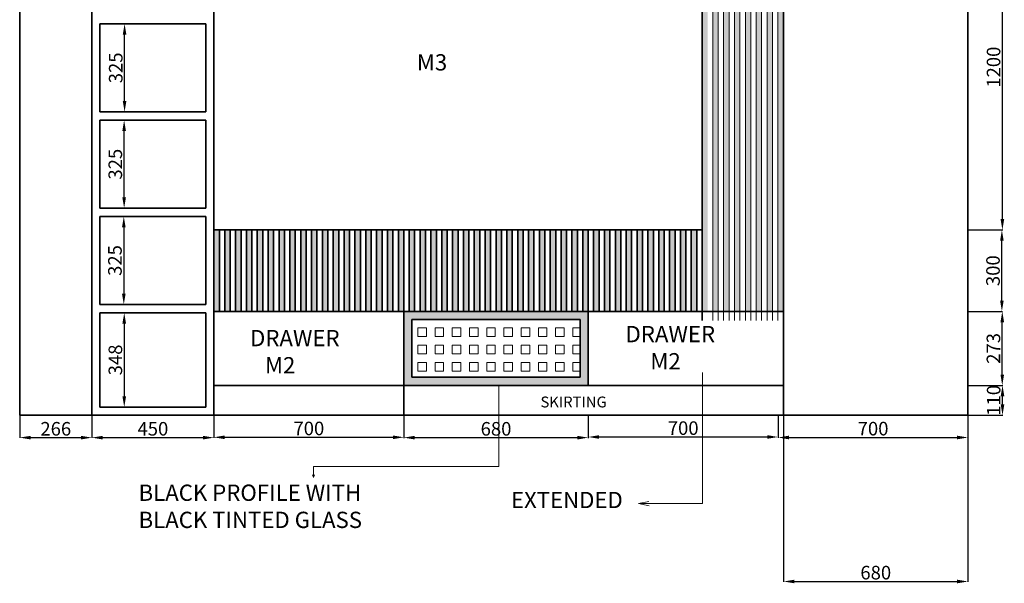
# Model space of a CAD drawing. Units: millimetres. Extents: x 11439 to 24661, y -4767 to -6.
# Tile 3 of 5: x 18965 to 22595, y -4767 to -2690. Entities that reach past the tile are written whole.
import ezdxf

# ---------------------------------------------------------------- set-up
doc = ezdxf.new("R2010")
doc.units = ezdxf.units.MM
for name, color, linetype, lineweight in [('A-ANNO-DIMS', 2, 'Continuous', 18), ('A-ANNO-TEXT', 3, 'Continuous', 18), ('A-FURN', 7, 'Continuous', 35), ('A-FURN-PATT', 8, 'Continuous', 13)]:
    doc.layers.add(name, color=color, linetype=linetype, lineweight=lineweight)
doc.styles.get("Standard").update_dxf_attribs({"font": 'arial.ttf'})
doc.dimstyles.new('ISO-25', dxfattribs={"dimtxt": 50, "dimasz": 40, "dimexe": 1.25, "dimexo": 0.625, "dimtad": 1, "dimtxsty": 'Standard', "dimcen": 2.5, "dimadec": 0, "dimazin": 0, "dimtfac": 1, "dimtmove": 0, "dimatfit": 3, "dimfxl": 1, "dimarcsym": 0})

# ---------------------------------------------------------------- blocks, each defined once
blk = doc.blocks.new('*D31')
at = {"layer": 'A-ANNO-DIMS', "color": 0, "lineweight": -2, "transparency": 16777216}
for p, q in [((18964.8, -4148.3), (18964.8, -4231.3)), ((19230.8, -4148.3), (19230.8, -4231.3)), ((19004.8, -4230), (19190.8, -4230))]:
    blk.add_line(p, q, dxfattribs=at)
at = {"layer": 'A-ANNO-DIMS', "color": 0, "transparency": 16777216}
for points in [[(19004.8, -4223.4), (19004.8, -4236.7), (18964.8, -4230)], [(19190.8, -4223.4), (19190.8, -4236.7), (19230.8, -4230)]]:
    blk.add_solid(points, dxfattribs=at)
at = {"layer": 'Defpoints', "color": 0, "transparency": 16777216}
for p in [(18964.8, -4147.7), (19230.8, -4147.7), (19230.8, -4230)]:
    blk.add_point(p, dxfattribs=at)
at = {"layer": 'A-ANNO-DIMS', "color": 0, "transparency": 16777216, "insert": (19097.8, -4203.9), "char_height": 50, "attachment_point": 5}
blk.add_mtext('266', dxfattribs=at)
blk = doc.blocks.new('*D32')
at = {"layer": 'A-ANNO-DIMS', "color": 0, "lineweight": -2, "transparency": 16777216}
for p, q in [((19230.8, -4148.3), (19230.8, -4231.3)), ((19680.8, -4148.3), (19680.8, -4231.3)), ((19270.8, -4230), (19640.8, -4230))]:
    blk.add_line(p, q, dxfattribs=at)
at = {"layer": 'A-ANNO-DIMS', "color": 0, "transparency": 16777216}
for points in [[(19270.8, -4223.4), (19270.8, -4236.7), (19230.8, -4230)], [(19640.8, -4223.4), (19640.8, -4236.7), (19680.8, -4230)]]:
    blk.add_solid(points, dxfattribs=at)
at = {"layer": 'Defpoints', "color": 0, "transparency": 16777216}
for p in [(19230.8, -4147.7), (19680.8, -4147.7), (19680.8, -4230)]:
    blk.add_point(p, dxfattribs=at)
at = {"layer": 'A-ANNO-DIMS', "color": 0, "transparency": 16777216, "insert": (19455.8, -4203.9), "char_height": 50, "attachment_point": 5}
blk.add_mtext('450', dxfattribs=at)
blk = doc.blocks.new('*D33')
at = {"layer": 'A-ANNO-DIMS', "color": 0, "lineweight": -2, "transparency": 16777216}
for p, q in [((19680.8, -4148.3), (19680.8, -4230.1)), ((20380.8, -4148.3), (20380.8, -4230.1)), ((19720.8, -4228.8), (20340.8, -4228.8))]:
    blk.add_line(p, q, dxfattribs=at)
at = {"layer": 'A-ANNO-DIMS', "color": 0, "transparency": 16777216}
for points in [[(19720.8, -4222.2), (19720.8, -4235.5), (19680.8, -4228.8)], [(20340.8, -4222.2), (20340.8, -4235.5), (20380.8, -4228.8)]]:
    blk.add_solid(points, dxfattribs=at)
at = {"layer": 'Defpoints', "color": 0, "transparency": 16777216}
for p in [(19680.8, -4147.7), (20380.8, -4147.7), (20380.8, -4228.8)]:
    blk.add_point(p, dxfattribs=at)
at = {"layer": 'A-ANNO-DIMS', "color": 0, "transparency": 16777216, "insert": (20030.8, -4202.7), "char_height": 50, "attachment_point": 5}
blk.add_mtext('700', dxfattribs=at)
blk = doc.blocks.new('*D34')
at = {"layer": 'A-ANNO-DIMS', "color": 0, "lineweight": -2, "transparency": 16777216}
for p, q in [((20380.8, -4148.3), (20380.8, -4231.4)), ((21060.8, -4148.3), (21060.8, -4231.4)), ((20420.8, -4230.1), (21020.8, -4230.1))]:
    blk.add_line(p, q, dxfattribs=at)
at = {"layer": 'A-ANNO-DIMS', "color": 0, "transparency": 16777216}
for points in [[(20420.8, -4223.5), (20420.8, -4236.8), (20380.8, -4230.1)], [(21020.8, -4223.5), (21020.8, -4236.8), (21060.8, -4230.1)]]:
    blk.add_solid(points, dxfattribs=at)
at = {"layer": 'Defpoints', "color": 0, "transparency": 16777216}
for p in [(20380.8, -4147.7), (21060.8, -4147.7), (21060.8, -4230.1)]:
    blk.add_point(p, dxfattribs=at)
at = {"layer": 'A-ANNO-DIMS', "color": 0, "transparency": 16777216, "insert": (20720.8, -4204), "char_height": 50, "attachment_point": 5}
blk.add_mtext('680', dxfattribs=at)
blk = doc.blocks.new('*D21')
at = {"layer": 'A-ANNO-DIMS', "color": 0, "lineweight": -2, "transparency": 16777216}
for p, q in [((21060.8, -4148.3), (21060.8, -4228.9)), ((21760.8, -4148.3), (21760.8, -4228.9)), ((21100.8, -4227.7), (21720.8, -4227.7))]:
    blk.add_line(p, q, dxfattribs=at)
at = {"layer": 'A-ANNO-DIMS', "color": 0, "transparency": 16777216}
for points in [[(21100.8, -4221), (21100.8, -4234.4), (21060.8, -4227.7)], [(21720.8, -4221), (21720.8, -4234.4), (21760.8, -4227.7)]]:
    blk.add_solid(points, dxfattribs=at)
at = {"layer": 'Defpoints', "color": 0, "transparency": 16777216}
for p in [(21060.8, -4147.7), (21760.8, -4147.7), (21760.8, -4227.7)]:
    blk.add_point(p, dxfattribs=at)
at = {"layer": 'A-ANNO-DIMS', "color": 0, "transparency": 16777216, "insert": (21410.8, -4201.5), "char_height": 50, "attachment_point": 5}
blk.add_mtext('700', dxfattribs=at)
blk = doc.blocks.new('*D35')
at = {"layer": 'A-ANNO-DIMS', "color": 0, "lineweight": -2, "transparency": 16777216}
for p, q in [((21760.8, -4148.3), (21760.8, -4230.8)), ((22460.8, -4148.3), (22460.8, -4230.8)), ((21800.8, -4229.6), (22420.8, -4229.6))]:
    blk.add_line(p, q, dxfattribs=at)
at = {"layer": 'A-ANNO-DIMS', "color": 0, "transparency": 16777216}
for points in [[(21800.8, -4222.9), (21800.8, -4236.3), (21760.8, -4229.6)], [(22420.8, -4222.9), (22420.8, -4236.3), (22460.8, -4229.6)]]:
    blk.add_solid(points, dxfattribs=at)
at = {"layer": 'Defpoints', "color": 0, "transparency": 16777216}
for p in [(21760.8, -4147.7), (22460.8, -4147.7), (22460.8, -4229.6)]:
    blk.add_point(p, dxfattribs=at)
at = {"layer": 'A-ANNO-DIMS', "color": 0, "transparency": 16777216, "insert": (22110.8, -4203.4), "char_height": 50, "attachment_point": 5}
blk.add_mtext('700', dxfattribs=at)
blk = doc.blocks.new('*D22')
at = {"layer": 'A-ANNO-DIMS', "color": 0, "lineweight": -2, "transparency": 16777216}
for p, q in [((22461.4, -4037.7), (22589.2, -4037.7)), ((22588, -4107.7), (22588, -4077.7)), ((22461.4, -4147.7), (22589.2, -4147.7))]:
    blk.add_line(p, q, dxfattribs=at)
at = {"layer": 'A-ANNO-DIMS', "color": 0, "transparency": 16777216}
for points in [[(22581.3, -4077.7), (22594.7, -4077.7), (22588, -4037.7)], [(22581.3, -4107.7), (22594.7, -4107.7), (22588, -4147.7)]]:
    blk.add_solid(points, dxfattribs=at)
at = {"layer": 'Defpoints', "color": 0, "transparency": 16777216}
for p in [(22460.8, -4037.7), (22588, -4037.7), (22460.8, -4147.7)]:
    blk.add_point(p, dxfattribs=at)
at = {"layer": 'A-ANNO-DIMS', "color": 0, "transparency": 16777216, "insert": (22561.8, -4092.7), "char_height": 50, "attachment_point": 5, "rotation": 90}
blk.add_mtext('110', dxfattribs=at)
blk = doc.blocks.new('*D26')
at = {"layer": 'A-ANNO-DIMS', "color": 0, "lineweight": -2, "transparency": 16777216}
for p, q in [((22461.4, -3764.7), (22588.4, -3764.7)), ((22587.1, -3997.7), (22587.1, -3804.7)), ((22461.4, -4037.7), (22588.4, -4037.7))]:
    blk.add_line(p, q, dxfattribs=at)
at = {"layer": 'A-ANNO-DIMS', "color": 0, "transparency": 16777216}
for points in [[(22580.5, -3804.7), (22593.8, -3804.7), (22587.1, -3764.7)], [(22580.5, -3997.7), (22593.8, -3997.7), (22587.1, -4037.7)]]:
    blk.add_solid(points, dxfattribs=at)
at = {"layer": 'Defpoints', "color": 0, "transparency": 16777216}
for p in [(22460.8, -3764.7), (22587.1, -3764.7), (22460.8, -4037.7)]:
    blk.add_point(p, dxfattribs=at)
at = {"layer": 'A-ANNO-DIMS', "color": 0, "transparency": 16777216, "insert": (22561, -3901.2), "char_height": 50, "attachment_point": 5, "rotation": 90}
blk.add_mtext('273', dxfattribs=at)
blk = doc.blocks.new('*D27')
at = {"layer": 'A-ANNO-DIMS', "color": 0, "lineweight": -2, "transparency": 16777216}
for p, q in [((22461.4, -3464.7), (22586.9, -3464.7)), ((22585.7, -3724.7), (22585.7, -3504.7)), ((22461.4, -3764.7), (22586.9, -3764.7))]:
    blk.add_line(p, q, dxfattribs=at)
at = {"layer": 'A-ANNO-DIMS', "color": 0, "transparency": 16777216}
for points in [[(22579, -3504.7), (22592.4, -3504.7), (22585.7, -3464.7)], [(22579, -3724.7), (22592.4, -3724.7), (22585.7, -3764.7)]]:
    blk.add_solid(points, dxfattribs=at)
at = {"layer": 'Defpoints', "color": 0, "transparency": 16777216}
for p in [(22460.8, -3464.7), (22585.7, -3464.7), (22460.8, -3764.7)]:
    blk.add_point(p, dxfattribs=at)
at = {"layer": 'A-ANNO-DIMS', "color": 0, "transparency": 16777216, "insert": (22559.5, -3614.7), "char_height": 50, "attachment_point": 5, "rotation": 90}
blk.add_mtext('300', dxfattribs=at)
blk = doc.blocks.new('*D28')
at = {"layer": 'A-ANNO-DIMS', "color": 0, "lineweight": -2, "transparency": 16777216}
for p, q in [((22461.4, -2264.7), (22588.9, -2264.7)), ((22587.6, -3424.7), (22587.6, -2304.7)), ((22461.4, -3464.7), (22588.9, -3464.7))]:
    blk.add_line(p, q, dxfattribs=at)
at = {"layer": 'A-ANNO-DIMS', "color": 0, "transparency": 16777216}
for points in [[(22581, -2304.7), (22594.3, -2304.7), (22587.6, -2264.7)], [(22581, -3424.7), (22594.3, -3424.7), (22587.6, -3464.7)]]:
    blk.add_solid(points, dxfattribs=at)
at = {"layer": 'Defpoints', "color": 0, "transparency": 16777216}
for p in [(22460.8, -2264.7), (22587.6, -2264.7), (22460.8, -3464.7)]:
    blk.add_point(p, dxfattribs=at)
at = {"layer": 'A-ANNO-DIMS', "color": 0, "transparency": 16777216, "insert": (22561.5, -2864.7), "char_height": 50, "attachment_point": 5, "rotation": 90}
blk.add_mtext('1200', dxfattribs=at)
blk = doc.blocks.new('*D37')
at = {"layer": 'A-ANNO-DIMS', "color": 0, "lineweight": -2, "transparency": 16777216}
for p, q in [((19455.1, -3769.7), (19348.9, -3769.7)), ((19350.2, -3809.7), (19350.2, -4077.7)), ((19455.1, -4117.7), (19348.9, -4117.7))]:
    blk.add_line(p, q, dxfattribs=at)
at = {"layer": 'A-ANNO-DIMS', "color": 0, "transparency": 16777216}
for points in [[(19343.5, -3809.7), (19356.8, -3809.7), (19350.2, -3769.7)], [(19343.5, -4077.7), (19356.8, -4077.7), (19350.2, -4117.7)]]:
    blk.add_solid(points, dxfattribs=at)
at = {"layer": 'Defpoints', "color": 0, "transparency": 16777216}
for p in [(19455.8, -3769.7), (19350.2, -4117.7), (19455.8, -4117.7)]:
    blk.add_point(p, dxfattribs=at)
at = {"layer": 'A-ANNO-DIMS', "color": 0, "transparency": 16777216, "insert": (19324, -3943.7), "char_height": 50, "attachment_point": 5, "rotation": 90}
blk.add_mtext('348', dxfattribs=at)
blk = doc.blocks.new('*D38')
at = {"layer": 'A-ANNO-DIMS', "color": 0, "lineweight": -2, "transparency": 16777216}
for p, q in [((19261.4, -3414.7), (19349.8, -3414.7)), ((19348.6, -3454.7), (19348.6, -3699.7)), ((19261.4, -3739.7), (19349.8, -3739.7))]:
    blk.add_line(p, q, dxfattribs=at)
at = {"layer": 'A-ANNO-DIMS', "color": 0, "transparency": 16777216}
for points in [[(19341.9, -3454.7), (19355.3, -3454.7), (19348.6, -3414.7)], [(19341.9, -3699.7), (19355.3, -3699.7), (19348.6, -3739.7)]]:
    blk.add_solid(points, dxfattribs=at)
at = {"layer": 'Defpoints', "color": 0, "transparency": 16777216}
for p in [(19260.8, -3414.7), (19260.8, -3739.7), (19348.6, -3739.7)]:
    blk.add_point(p, dxfattribs=at)
at = {"layer": 'A-ANNO-DIMS', "color": 0, "transparency": 16777216, "insert": (19322.4, -3577.2), "char_height": 50, "attachment_point": 5, "rotation": 90}
blk.add_mtext('325', dxfattribs=at)
blk = doc.blocks.new('*D39')
at = {"layer": 'A-ANNO-DIMS', "color": 0, "lineweight": -2, "transparency": 16777216}
for p, q in [((19261.4, -3059.7), (19351.1, -3059.7)), ((19349.8, -3344.7), (19349.8, -3099.7)), ((19261.4, -3384.7), (19351.1, -3384.7))]:
    blk.add_line(p, q, dxfattribs=at)
at = {"layer": 'A-ANNO-DIMS', "color": 0, "transparency": 16777216}
for points in [[(19343.2, -3099.7), (19356.5, -3099.7), (19349.8, -3059.7)], [(19343.2, -3344.7), (19356.5, -3344.7), (19349.8, -3384.7)]]:
    blk.add_solid(points, dxfattribs=at)
at = {"layer": 'Defpoints', "color": 0, "transparency": 16777216}
for p in [(19260.8, -3059.7), (19349.8, -3059.7), (19260.8, -3384.7)]:
    blk.add_point(p, dxfattribs=at)
at = {"layer": 'A-ANNO-DIMS', "color": 0, "transparency": 16777216, "insert": (19323.7, -3222.2), "char_height": 50, "attachment_point": 5, "rotation": 90}
blk.add_mtext('325', dxfattribs=at)
blk = doc.blocks.new('*D40')
at = {"layer": 'A-ANNO-DIMS', "color": 0, "lineweight": -2, "transparency": 16777216}
for p, q in [((19261.4, -2704.7), (19352.7, -2704.7)), ((19351.5, -2989.7), (19351.5, -2744.7)), ((19261.4, -3029.7), (19352.7, -3029.7))]:
    blk.add_line(p, q, dxfattribs=at)
at = {"layer": 'A-ANNO-DIMS', "color": 0, "transparency": 16777216}
for points in [[(19344.8, -2744.7), (19358.1, -2744.7), (19351.5, -2704.7)], [(19344.8, -2989.7), (19358.1, -2989.7), (19351.5, -3029.7)]]:
    blk.add_solid(points, dxfattribs=at)
at = {"layer": 'Defpoints', "color": 0, "transparency": 16777216}
for p in [(19260.8, -2704.7), (19351.5, -2704.7), (19260.8, -3029.7)]:
    blk.add_point(p, dxfattribs=at)
at = {"layer": 'A-ANNO-DIMS', "color": 0, "transparency": 16777216, "insert": (19325.3, -2867.2), "char_height": 50, "attachment_point": 5, "rotation": 90}
blk.add_mtext('325', dxfattribs=at)
blk = doc.blocks.new('SHELF-COMPARTMENT')
for p, q in [((0, 325), (390, 325)), ((0, 0), (0, 325)), ((390, 0), (390, 325)), ((0, 0), (390, 0))]:
    blk.add_line(p, q)
blk = doc.blocks.new('DRAWER-GLASS-FRONT')
for p, q in [((0, 213), (620, 213)), ((0, 0), (0, 213)), ((620, 0), (620, 213)), ((0, 0), (620, 0))]:
    blk.add_line(p, q)
blk = doc.blocks.new('*D59')
at = {"layer": 'A-ANNO-DIMS', "color": 0, "lineweight": -2, "transparency": 16777216}
for p, q in [((21780.8, -4148.3), (21780.8, -4761.5)), ((22460.8, -4148.3), (22460.8, -4761.5)), ((21820.8, -4760.3), (22420.8, -4760.3))]:
    blk.add_line(p, q, dxfattribs=at)
at = {"layer": 'A-ANNO-DIMS', "color": 0, "transparency": 16777216}
for points in [[(21820.8, -4753.6), (21820.8, -4766.9), (21780.8, -4760.3)], [(22420.8, -4753.6), (22420.8, -4766.9), (22460.8, -4760.3)]]:
    blk.add_solid(points, dxfattribs=at)
at = {"layer": 'Defpoints', "color": 0, "transparency": 16777216}
for p in [(21780.8, -4147.7), (22460.8, -4147.7), (22460.8, -4760.3)]:
    blk.add_point(p, dxfattribs=at)
at = {"layer": 'A-ANNO-DIMS', "color": 0, "transparency": 16777216, "insert": (22120.8, -4734.1), "char_height": 50, "attachment_point": 5}
blk.add_mtext('680', dxfattribs=at)

msp = doc.modelspace()

# ---------------------------------------------------------------- hatches: boundary and pattern name
at = {"layer": 'A-FURN-PATT'}
h = msp.add_hatch(color=256, dxfattribs=at)
h.dxf.hatch_style = 1
h.paths.add_polyline_path([(19700.761, -3464.684), (19680.761, -3464.684), (19680.761, -3764.684), (19700.761, -3764.684)])
h.paths.add_polyline_path([(19740.761, -3464.684), (19720.761, -3464.684), (19720.761, -3764.684), (19740.761, -3764.684)])
h.paths.add_polyline_path([(19780.761, -3464.684), (19760.761, -3464.684), (19760.761, -3764.684), (19780.761, -3764.684)])
h.paths.add_polyline_path([(19800.761, -3764.684), (19820.761, -3764.684), (19820.761, -3464.684), (19800.761, -3464.684)])
h.paths.add_polyline_path([(19860.761, -3464.684), (19840.761, -3464.684), (19840.761, -3764.684), (19860.761, -3764.684)])
h.paths.add_polyline_path([(19900.761, -3464.684), (19880.761, -3464.684), (19880.761, -3764.684), (19900.761, -3764.684)])
h.paths.add_polyline_path([(19940.761, -3464.684), (19920.761, -3464.684), (19920.761, -3764.684), (19940.761, -3764.684)])
h.paths.add_polyline_path([(19960.761, -3764.684), (19980.761, -3764.684), (19980.761, -3464.684), (19960.761, -3464.684)])
h.paths.add_polyline_path([(20020.761, -3464.684), (20000.761, -3464.684), (20000.761, -3764.684), (20020.761, -3764.684)])
h.paths.add_polyline_path([(20040.761, -3764.684), (20060.761, -3764.684), (20060.761, -3464.684), (20040.761, -3464.684)])
h.paths.add_polyline_path([(20080.761, -3764.684), (20100.761, -3764.684), (20100.761, -3464.684), (20080.761, -3464.684)])
h.paths.add_polyline_path([(20140.761, -3464.684), (20120.761, -3464.684), (20120.761, -3764.684), (20140.761, -3764.684)])
h.paths.add_polyline_path([(20160.761, -3764.684), (20180.761, -3764.684), (20180.761, -3464.684), (20160.761, -3464.684)])
h.paths.add_polyline_path([(20220.761, -3464.684), (20200.761, -3464.684), (20200.761, -3764.684), (20220.761, -3764.684)])
h.paths.add_polyline_path([(20240.761, -3764.684), (20260.761, -3764.684), (20260.761, -3464.684), (20240.761, -3464.684)])
h.paths.add_polyline_path([(20300.761, -3464.684), (20280.761, -3464.684), (20280.761, -3764.684), (20300.761, -3764.684)])
h.paths.add_polyline_path([(20340.761, -3464.684), (20320.761, -3464.684), (20320.761, -3764.684), (20340.761, -3764.684)])
h.paths.add_polyline_path([(20360.761, -3764.684), (20380.761, -3764.684), (20380.761, -3464.684), (20360.761, -3464.684)])
h.paths.add_polyline_path([(20400.761, -3764.684), (20420.761, -3764.684), (20420.761, -3464.684), (20400.761, -3464.684)])
h.paths.add_polyline_path([(20440.761, -3764.684), (20460.761, -3764.684), (20460.761, -3464.684), (20440.761, -3464.684)])
h.paths.add_polyline_path([(20480.761, -3764.684), (20500.761, -3764.684), (20500.761, -3464.684), (20480.761, -3464.684)])
h.paths.add_polyline_path([(20520.761, -3764.684), (20540.761, -3764.684), (20540.761, -3464.684), (20520.761, -3464.684)])
h.paths.add_polyline_path([(20560.761, -3764.684), (20580.761, -3764.684), (20580.761, -3464.684), (20560.761, -3464.684)])
h.paths.add_polyline_path([(20600.761, -3764.684), (20620.761, -3764.684), (20620.761, -3464.684), (20600.761, -3464.684)])
h.paths.add_polyline_path([(20660.761, -3464.684), (20640.761, -3464.684), (20640.761, -3764.684), (20660.761, -3764.684)])
h.paths.add_polyline_path([(20680.761, -3764.684), (20700.761, -3764.684), (20700.761, -3464.684), (20680.761, -3464.684)])
h.paths.add_polyline_path([(20740.761, -3464.684), (20720.761, -3464.684), (20720.761, -3764.684), (20740.761, -3764.684)])
h.paths.add_polyline_path([(20760.761, -3764.684), (20780.761, -3764.684), (20780.761, -3464.684), (20760.761, -3464.684)])
h.paths.add_polyline_path([(20800.761, -3764.684), (20820.761, -3764.684), (20820.761, -3464.684), (20800.761, -3464.684)])
h.paths.add_polyline_path([(20840.761, -3764.684), (20860.761, -3764.684), (20860.761, -3464.684), (20840.761, -3464.684)])
h.paths.add_polyline_path([(20900.761, -3464.684), (20880.761, -3464.684), (20880.761, -3764.684), (20900.761, -3764.684)])
h.paths.add_polyline_path([(20940.761, -3464.684), (20920.761, -3464.684), (20920.761, -3764.684), (20940.761, -3764.684)])
h.paths.add_polyline_path([(20980.761, -3464.684), (20960.761, -3464.684), (20960.761, -3764.684), (20980.761, -3764.684)])
h.paths.add_polyline_path([(21020.761, -3464.684), (21000.761, -3464.684), (21000.761, -3764.684), (21020.761, -3764.684)])
h.paths.add_polyline_path([(21060.761, -3464.684), (21040.761, -3464.684), (21040.761, -3764.684), (21060.761, -3764.684)])
h.paths.add_polyline_path([(21080.761, -3764.684), (21100.761, -3764.684), (21100.761, -3464.684), (21080.761, -3464.684)])
h.paths.add_polyline_path([(21120.761, -3764.684), (21140.761, -3764.684), (21140.761, -3464.684), (21120.761, -3464.684)])
h.paths.add_polyline_path([(21180.761, -3464.684), (21160.761, -3464.684), (21160.761, -3764.684), (21180.761, -3764.684)])
h.paths.add_polyline_path([(21200.761, -3764.684), (21220.761, -3764.684), (21220.761, -3464.684), (21200.761, -3464.684)])
h.paths.add_polyline_path([(21260.761, -3464.684), (21240.761, -3464.684), (21240.761, -3764.684), (21260.761, -3764.684)])
h.paths.add_polyline_path([(21280.761, -3764.684), (21300.761, -3764.684), (21300.761, -3464.684), (21280.761, -3464.684)])
h.paths.add_polyline_path([(21320.761, -3764.684), (21340.761, -3764.684), (21340.761, -3464.684), (21320.761, -3464.684)])
h.paths.add_polyline_path([(21360.761, -3764.684), (21380.761, -3764.684), (21380.761, -3464.684), (21360.761, -3464.684)])
h.paths.add_polyline_path([(21400.761, -3764.684), (21420.761, -3764.684), (21420.761, -3464.684), (21400.761, -3464.684)])
h.paths.add_polyline_path([(21460.761, -3464.684), (21440.761, -3464.684), (21440.761, -3764.684), (21460.761, -3764.684)])
h.paths.add_polyline_path([(19700.761, -1964.684), (19680.761, -1964.684), (19680.761, -2264.684), (19700.761, -2264.684)])
h.paths.add_polyline_path([(19740.761, -1964.684), (19720.761, -1964.684), (19720.761, -2264.684), (19740.761, -2264.684)])
h.paths.add_polyline_path([(19780.761, -1964.684), (19760.761, -1964.684), (19760.761, -2264.684), (19780.761, -2264.684)])
h.paths.add_polyline_path([(19820.761, -1964.684), (19800.761, -1964.684), (19800.761, -2264.684), (19820.761, -2264.684)])
h.paths.add_polyline_path([(19860.761, -2264.684), (19860.761, -1964.684), (19840.761, -1964.684), (19840.761, -2264.684)])
h.paths.add_polyline_path([(19880.761, -2264.684), (19900.761, -2264.684), (19900.761, -1964.684), (19880.761, -1964.684)])
h.paths.add_polyline_path([(19940.761, -1964.684), (19920.761, -1964.684), (19920.761, -2264.684), (19940.761, -2264.684)])
h.paths.add_polyline_path([(19960.761, -2264.684), (19980.761, -2264.684), (19980.761, -1964.684), (19960.761, -1964.684)])
h.paths.add_polyline_path([(20020.761, -1964.684), (20000.761, -1964.684), (20000.761, -2264.684), (20020.761, -2264.684)])
h.paths.add_polyline_path([(20040.761, -2264.684), (20060.761, -2264.684), (20060.761, -1964.684), (20040.761, -1964.684)])
h.paths.add_polyline_path([(20100.761, -1964.684), (20080.761, -1964.684), (20080.761, -2264.684), (20100.761, -2264.684)])
h.paths.add_polyline_path([(20120.761, -2264.684), (20140.761, -2264.684), (20140.761, -1964.684), (20120.761, -1964.684)])
h.paths.add_polyline_path([(20180.761, -1964.684), (20160.761, -1964.684), (20160.761, -2264.684), (20180.761, -2264.684)])
h.paths.add_polyline_path([(20220.761, -1964.684), (20200.761, -1964.684), (20200.761, -2264.684), (20220.761, -2264.684)])
h.paths.add_polyline_path([(20240.761, -2264.684), (20260.761, -2264.684), (20260.761, -1964.684), (20240.761, -1964.684)])
h.paths.add_polyline_path([(20280.761, -2264.684), (20300.761, -2264.684), (20300.761, -1964.684), (20280.761, -1964.684)])
h.paths.add_polyline_path([(20340.761, -1964.684), (20320.761, -1964.684), (20320.761, -2264.684), (20340.761, -2264.684)])
h.paths.add_polyline_path([(20360.761, -2264.684), (20380.761, -2264.684), (20380.761, -1964.684), (20360.761, -1964.684)])
h.paths.add_polyline_path([(20400.761, -2264.684), (20420.761, -2264.684), (20420.761, -1964.684), (20400.761, -1964.684)])
h.paths.add_polyline_path([(20440.761, -2264.684), (20460.761, -2264.684), (20460.761, -1964.684), (20440.761, -1964.684)])
h.paths.add_polyline_path([(20480.761, -2264.684), (20500.761, -2264.684), (20500.761, -1964.684), (20480.761, -1964.684)])
h.paths.add_polyline_path([(20520.761, -2264.684), (20540.761, -2264.684), (20540.761, -1964.684), (20520.761, -1964.684)])
h.paths.add_polyline_path([(20580.761, -1964.684), (20560.761, -1964.684), (20560.761, -2264.684), (20580.761, -2264.684)])
h.paths.add_polyline_path([(20600.761, -2264.684), (20620.761, -2264.684), (20620.761, -1964.684), (20600.761, -1964.684)])
h.paths.add_polyline_path([(20640.761, -2264.684), (20660.761, -2264.684), (20660.761, -1964.684), (20640.761, -1964.684)])
h.paths.add_polyline_path([(20680.761, -2264.684), (20700.761, -2264.684), (20700.761, -1964.684), (20680.761, -1964.684)])
h.paths.add_polyline_path([(20720.761, -2264.684), (20740.761, -2264.684), (20740.761, -1964.684), (20720.761, -1964.684)])
h.paths.add_polyline_path([(20780.761, -1964.684), (20760.761, -1964.684), (20760.761, -2264.684), (20780.761, -2264.684)])
h.paths.add_polyline_path([(20800.761, -2264.684), (20820.761, -2264.684), (20820.761, -1964.684), (20800.761, -1964.684)])
h.paths.add_polyline_path([(20860.761, -1964.684), (20840.761, -1964.684), (20840.761, -2264.684), (20860.761, -2264.684)])
h.paths.add_polyline_path([(20900.761, -1964.684), (20880.761, -1964.684), (20880.761, -2264.684), (20900.761, -2264.684)])
h.paths.add_polyline_path([(20940.761, -1964.684), (20920.761, -1964.684), (20920.761, -2264.684), (20940.761, -2264.684)])
h.paths.add_polyline_path([(20980.761, -1964.684), (20960.761, -1964.684), (20960.761, -2264.684), (20980.761, -2264.684)])
h.paths.add_polyline_path([(21020.761, -1964.684), (21000.761, -1964.684), (21000.761, -2264.684), (21020.761, -2264.684)])
h.paths.add_polyline_path([(21040.761, -2264.684), (21060.761, -2264.684), (21060.761, -1964.684), (21040.761, -1964.684)])
h.paths.add_polyline_path([(21080.761, -2264.684), (21100.761, -2264.684), (21100.761, -1964.684), (21080.761, -1964.684)])
h.paths.add_polyline_path([(21120.761, -2264.684), (21140.761, -2264.684), (21140.761, -1964.684), (21120.761, -1964.684)])
h.paths.add_polyline_path([(21180.761, -1964.684), (21160.761, -1964.684), (21160.761, -2264.684), (21180.761, -2264.684)])
h.paths.add_polyline_path([(21200.761, -2264.684), (21220.761, -2264.684), (21220.761, -1964.684), (21200.761, -1964.684)])
h.paths.add_polyline_path([(21240.761, -2264.684), (21260.761, -2264.684), (21260.761, -1964.684), (21240.761, -1964.684)])
h.paths.add_polyline_path([(21300.761, -1964.684), (21280.761, -1964.684), (21280.761, -2264.684), (21300.761, -2264.684)])
h.paths.add_polyline_path([(21320.761, -2264.684), (21340.761, -2264.684), (21340.761, -1964.684), (21320.761, -1964.684)])
h.paths.add_polyline_path([(21360.761, -2264.684), (21380.761, -2264.684), (21380.761, -1964.684), (21360.761, -1964.684)])
h.paths.add_polyline_path([(21400.761, -2264.684), (21420.761, -2264.684), (21420.761, -1964.684), (21400.761, -1964.684)])
h.paths.add_polyline_path([(21440.761, -2264.684), (21460.761, -2264.684), (21460.761, -1964.684), (21440.761, -1964.684)])
h = msp.add_hatch(color=256, dxfattribs=at)
h.dxf.hatch_style = 1
h.paths.add_polyline_path([(21500.761, -2881.594), (21480.761, -2881.594), (21480.761, -3464.684), (21480.761, -3764.684), (21500.761, -3764.684)])
h.paths.add_polyline_path([(21540.761, -2881.594), (21520.761, -2881.594), (21520.761, -3764.684), (21540.761, -3764.684)])
h.paths.add_polyline_path([(21580.761, -2881.594), (21560.761, -2881.594), (21560.761, -3764.684), (21580.761, -3764.684)])
h.paths.add_polyline_path([(21620.761, -2881.594), (21600.761, -2881.594), (21600.761, -3764.684), (21620.761, -3764.684)])
h.paths.add_polyline_path([(21660.761, -2881.594), (21640.761, -2881.594), (21640.761, -3764.684), (21660.761, -3764.684)])
h.paths.add_polyline_path([(21700.761, -2881.594), (21680.761, -2881.594), (21680.761, -3764.684), (21700.761, -3764.684)])
h.paths.add_polyline_path([(21740.761, -2881.594), (21720.761, -2881.594), (21720.761, -3764.684), (21740.761, -3764.684)])
h.paths.add_polyline_path([(21780.761, -2881.594), (21760.761, -2881.594), (21760.761, -3764.684), (21780.761, -3764.684)])
h.paths.add_polyline_path([(21500.761, -1964.684), (21480.761, -1964.684), (21480.761, -2264.684), (21480.761, -2881.594), (21500.761, -2881.594)])
h.paths.add_polyline_path([(21540.761, -1964.684), (21520.761, -1964.684), (21520.761, -2881.594), (21540.761, -2881.594)])
h.paths.add_polyline_path([(21580.761, -2095.642), (21560.761, -2095.642), (21560.761, -2881.594), (21580.761, -2881.594)])
h.paths.add_polyline_path([(21620.761, -2095.642), (21600.761, -2095.642), (21600.761, -2881.594), (21620.761, -2881.594)])
h.paths.add_polyline_path([(21660.761, -2095.642), (21640.761, -2095.642), (21640.761, -2881.594), (21660.761, -2881.594)])
h.paths.add_polyline_path([(21700.761, -2095.642), (21680.761, -2095.642), (21680.761, -2881.594), (21700.761, -2881.594)])
h.paths.add_polyline_path([(21740.761, -2095.642), (21720.761, -2095.642), (21720.761, -2881.594), (21740.761, -2881.594)])
h.paths.add_polyline_path([(21780.761, -2095.642), (21760.761, -2095.642), (21760.761, -2881.594), (21780.761, -2881.594)])
h = msp.add_hatch(dxfattribs=at)
h.set_pattern_fill('ANSI31', color=256, scale=6.29921, angle=45, style=0)
h.paths.add_polyline_path([(21500.761, -3798.504), (21760.761, -3798.504), (21760.761, -1964.684), (21500.761, -1964.684)])
h = msp.add_hatch(color=256, dxfattribs=at)
h.dxf.hatch_style = 1
h.paths.add_polyline_path([(21060.761, -4037.684), (21060.761, -3764.684), (20380.761, -3764.684), (20380.761, -4037.684)])
h.paths.add_polyline_path([(20410.761, -4007.684), (20410.761, -3794.684), (21030.761, -3794.684), (21030.761, -4007.684)], flags=16)
h = msp.add_hatch(dxfattribs=at)
h.set_pattern_fill('SQUARE', color=256, scale=10)
h.set_pattern_definition([(0, (5255.846, -47.69), (0, 31.75), [31.75, -31.75]), (90, (5255.846, -47.69), (-31.75, 2e-15), [31.75, -31.75])])
h.paths.add_polyline_path([(21030.761, -3794.684), (20410.761, -3794.684), (20410.761, -4007.684), (21030.761, -4007.684)])

# ---------------------------------------------------------------- linework, layer by layer
at = {"layer": 'A-ANNO-TEXT'}
for p, q in [((21482.07, -3989.814), (21482.07, -4473.399)), ((20730.761, -4037.684), (20730.761, -4336.93)), ((20730.761, -4336.93), (20047.978, -4336.93)), ((20047.978, -4336.93), (20047.978, -4377.58)), ((20047.978, -4377.58), (20044.568, -4366.993)), ((20047.978, -4377.58), (20051.243, -4367.31)), ((21245.532, -4473.399), (21284.053, -4465.608)), ((21482.07, -4473.399), (21245.532, -4473.399)), ((21245.532, -4473.399), (21285.168, -4481.76))]:
    msp.add_line(p, q, dxfattribs=at)
at = {"layer": 'A-FURN'}
for p, q in [((18964.761, -1337.684), (18964.761, -4147.684)), ((22460.761, -4147.684), (22460.761, -1337.684)), ((19230.761, -4147.684), (19230.761, -1964.684)), ((19680.761, -4147.684), (19680.761, -1964.684)), ((21780.761, -4147.684), (21780.761, -1964.684)), ((21480.761, -3464.684), (21480.761, -2264.684)), ((19680.761, -3464.684), (21480.761, -3464.684)), ((19700.761, -3764.684), (19700.761, -3464.684)), ((19720.761, -3764.684), (19720.761, -3464.684)), ((19740.761, -3764.684), (19740.761, -3464.684)), ((19760.761, -3764.684), (19760.761, -3464.684)), ((19780.761, -3764.684), (19780.761, -3464.684)), ((19800.761, -3764.684), (19800.761, -3464.684)), ((19820.761, -3764.684), (19820.761, -3464.684)), ((19840.761, -3764.684), (19840.761, -3464.684)), ((19860.761, -3764.684), (19860.761, -3464.684)), ((19880.761, -3764.684), (19880.761, -3464.684)), ((19900.761, -3764.684), (19900.761, -3464.684)), ((19920.761, -3764.684), (19920.761, -3464.684)), ((19940.761, -3764.684), (19940.761, -3464.684)), ((19960.761, -3764.684), (19960.761, -3464.684)), ((19980.761, -3764.684), (19980.761, -3464.684)), ((20000.761, -3764.684), (20000.761, -3464.684)), ((20020.761, -3764.684), (20020.761, -3464.684)), ((20040.761, -3764.684), (20040.761, -3464.684)), ((20060.761, -3764.684), (20060.761, -3464.684)), ((20080.761, -3764.684), (20080.761, -3464.684)), ((20100.761, -3764.684), (20100.761, -3464.684)), ((20120.761, -3764.684), (20120.761, -3464.684)), ((20140.761, -3764.684), (20140.761, -3464.684)), ((20160.761, -3764.684), (20160.761, -3464.684)), ((20180.761, -3764.684), (20180.761, -3464.684)), ((20200.761, -3764.684), (20200.761, -3464.684)), ((20220.761, -3764.684), (20220.761, -3464.684)), ((20240.761, -3764.684), (20240.761, -3464.684)), ((20260.761, -3764.684), (20260.761, -3464.684)), ((20280.761, -3764.684), (20280.761, -3464.684)), ((20300.761, -3764.684), (20300.761, -3464.684)), ((20320.761, -3764.684), (20320.761, -3464.684)), ((20340.761, -3764.684), (20340.761, -3464.684)), ((20360.761, -3764.684), (20360.761, -3464.684)), ((20380.761, -3764.684), (20380.761, -3464.684)), ((20400.761, -3764.684), (20400.761, -3464.684)), ((20420.761, -3764.684), (20420.761, -3464.684)), ((20440.761, -3764.684), (20440.761, -3464.684)), ((20460.761, -3764.684), (20460.761, -3464.684)), ((20480.761, -3764.684), (20480.761, -3464.684)), ((20500.761, -3764.684), (20500.761, -3464.684)), ((20520.761, -3764.684), (20520.761, -3464.684)), ((20540.761, -3764.684), (20540.761, -3464.684)), ((20560.761, -3764.684), (20560.761, -3464.684)), ((20580.761, -3764.684), (20580.761, -3464.684)), ((20600.761, -3764.684), (20600.761, -3464.684)), ((20620.761, -3764.684), (20620.761, -3464.684)), ((20640.761, -3764.684), (20640.761, -3464.684)), ((20660.761, -3764.684), (20660.761, -3464.684)), ((20680.761, -3764.684), (20680.761, -3464.684)), ((20700.761, -3764.684), (20700.761, -3464.684)), ((20720.761, -3764.684), (20720.761, -3464.684)), ((20740.761, -3764.684), (20740.761, -3464.684)), ((20760.761, -3764.684), (20760.761, -3464.684)), ((20780.761, -3764.684), (20780.761, -3464.684)), ((20800.761, -3764.684), (20800.761, -3464.684)), ((20820.761, -3764.684), (20820.761, -3464.684)), ((20840.761, -3764.684), (20840.761, -3464.684)), ((20860.761, -3764.684), (20860.761, -3464.684)), ((20880.761, -3764.684), (20880.761, -3464.684)), ((20900.761, -3764.684), (20900.761, -3464.684)), ((20920.761, -3764.684), (20920.761, -3464.684)), ((20940.761, -3764.684), (20940.761, -3464.684)), ((20960.761, -3764.684), (20960.761, -3464.684)), ((20980.761, -3764.684), (20980.761, -3464.684)), ((21000.761, -3764.684), (21000.761, -3464.684)), ((21020.761, -3764.684), (21020.761, -3464.684)), ((21040.761, -3764.684), (21040.761, -3464.684)), ((21060.761, -3764.684), (21060.761, -3464.684)), ((21080.761, -3764.684), (21080.761, -3464.684)), ((21100.761, -3764.684), (21100.761, -3464.684)), ((21120.761, -3764.684), (21120.761, -3464.684)), ((21140.761, -3764.684), (21140.761, -3464.684)), ((21160.761, -3764.684), (21160.761, -3464.684)), ((21180.761, -3764.684), (21180.761, -3464.684)), ((21200.761, -3764.684), (21200.761, -3464.684)), ((21220.761, -3764.684), (21220.761, -3464.684)), ((21240.761, -3764.684), (21240.761, -3464.684)), ((21260.761, -3764.684), (21260.761, -3464.684)), ((21280.761, -3764.684), (21280.761, -3464.684)), ((21300.761, -3764.684), (21300.761, -3464.684)), ((21320.761, -3764.684), (21320.761, -3464.684)), ((21340.761, -3764.684), (21340.761, -3464.684)), ((21360.761, -3764.684), (21360.761, -3464.684)), ((21380.761, -3764.684), (21380.761, -3464.684)), ((21400.761, -3764.684), (21400.761, -3464.684)), ((21420.761, -3764.684), (21420.761, -3464.684)), ((21440.761, -3764.684), (21440.761, -3464.684)), ((21460.761, -3764.684), (21460.761, -3464.684)), ((21480.761, -3464.684), (21480.761, -3798.504)), ((19260.761, -4117.684), (19260.761, -3769.684)), ((19260.761, -3769.684), (19650.761, -3769.684)), ((19650.761, -4117.684), (19650.761, -3769.684)), ((19680.761, -3764.684), (21780.761, -3764.684)), ((20380.761, -4147.684), (20380.761, -3764.684)), ((21060.761, -4037.684), (21060.761, -3764.684)), ((19680.761, -4037.684), (21780.761, -4037.684)), ((19260.761, -4117.684), (19650.761, -4117.684)), ((18964.761, -4147.684), (22460.761, -4147.684))]:
    msp.add_line(p, q, dxfattribs=at)

# ---------------------------------------------------------------- block references
at = {"layer": 'A-FURN', "rotation": 180}
for name, p in [('SHELF-COMPARTMENT', (19650.761, -2704.685)), ('SHELF-COMPARTMENT', (19650.761, -3059.685)), ('SHELF-COMPARTMENT', (19650.761, -3414.685)), ('DRAWER-GLASS-FRONT', (21030.76, -3794.685))]:
    msp.add_blockref(name, p, dxfattribs=at)

# ---------------------------------------------------------------- texts
at = {"layer": 'A-ANNO-TEXT', "attachment_point": 1}
for s, insert, char_height in [('\\P    M3', (20355.532, -2716.835), 60), (' DRAWER\\P    M2', (19795.718, -3833.205), 60), (' DRAWER \\P      M2', (21179.968, -3818.504), 60), ('SKIRTING ', (20884.725, -4078.649), 40), (' BLACK PROFILE WITH\\P BLACK TINTED GLASS', (19384.746, -4403.147), 60), ('EXTENDED', (20775.841, -4429.883), 60)]:
    msp.add_mtext_dynamic_manual_height_columns(s, width=1074.7282, gutter_width=12.5, heights=[0], dxfattribs=dict(at, insert=insert, char_height=char_height))

# ---------------------------------------------------------------- dimensions: what is measured, and where the dimension line sits
at = {"layer": 'A-ANNO-DIMS'}
for base, p1, p2, picture, middle in [((22587.626, -2264.684), (22460.761, -3464.684), (22460.761, -2264.684), '*D28', (22561.472, -2864.684)), ((19351.477, -2704.684), (19260.761, -3029.684), (19260.761, -2704.684), '*D40', (19325.306, -2867.184)), ((19349.845, -3059.684), (19260.761, -3384.684), (19260.761, -3059.684), '*D39', (19323.675, -3222.184)), ((19348.585, -3739.684), (19260.761, -3414.684), (19260.761, -3739.684), '*D38', (19322.415, -3577.184)), ((22585.7, -3464.684), (22460.761, -3764.684), (22460.761, -3464.684), '*D27', (22559.529, -3614.684)), ((19350.181, -4117.684), (19455.761, -3769.684), (19455.761, -4117.684), '*D37', (19324.01, -3943.684)), ((22587.135, -3764.684), (22460.761, -4037.684), (22460.761, -3764.684), '*D26', (22560.964, -3901.184)), ((22587.988, -4037.684), (22460.761, -4147.684), (22460.761, -4037.684), '*D22', (22561.835, -4092.684))]:
    dim = msp.add_linear_dim(base=base, p1=p1, p2=p2, angle=90, dimstyle='ISO-25', override={"dimclrd": 0, "dimclre": 0, "dimclrt": 0}, dxfattribs=at)
    dim.commit()
    dim.dimension.update_dxf_attribs({"geometry": picture, "text_midpoint": middle})
for base, p1, p2, override, picture, middle in [((19230.761, -4230.031), (18964.761, -4147.684), (19230.761, -4147.684), {"dimclrd": 0, "dimclre": 0, "dimclrt": 0}, '*D31', (19097.761, -4203.877)), ((19680.761, -4230.031), (19230.761, -4147.684), (19680.761, -4147.684), {"dimclrd": 0, "dimclre": 0, "dimclrt": 0}, '*D32', (19455.761, -4203.877)), ((20380.761, -4228.839), (19680.761, -4147.684), (20380.761, -4147.684), {"dimclrd": 0, "dimclre": 0, "dimclrt": 0}, '*D33', (20030.761, -4202.686)), ((21060.761, -4230.128), (20380.761, -4147.684), (21060.761, -4147.684), {"dimclrd": 0, "dimclre": 0, "dimclrt": 0}, '*D34', (20720.761, -4203.975)), ((21760.761, -4227.692), (21060.761, -4147.684), (21760.761, -4147.684), {"dimclrd": 0, "dimclre": 0, "dimclrt": 0}, '*D21', (21410.761, -4201.538)), ((22460.761, -4229.587), (21760.761, -4147.684), (22460.761, -4147.684), {"dimclrd": 0, "dimclre": 0, "dimclrt": 0}, '*D35', (22110.761, -4203.433)), ((22460.761, -4760.26), (21780.761, -4147.684), (22460.761, -4147.684), {"dimdec": 0, "dimlfac": 1, "dimrnd": 0, "dimzin": 0, "dimdsep": 46, "dimlunit": 2}, '*D59', (22120.761, -4734.106))]:
    dim = msp.add_linear_dim(base=base, p1=p1, p2=p2, dimstyle='ISO-25', override=override, dxfattribs=at)
    dim.commit()
    dim.dimension.update_dxf_attribs({"geometry": picture, "text_midpoint": middle})

doc.saveas('drawing.dxf')
